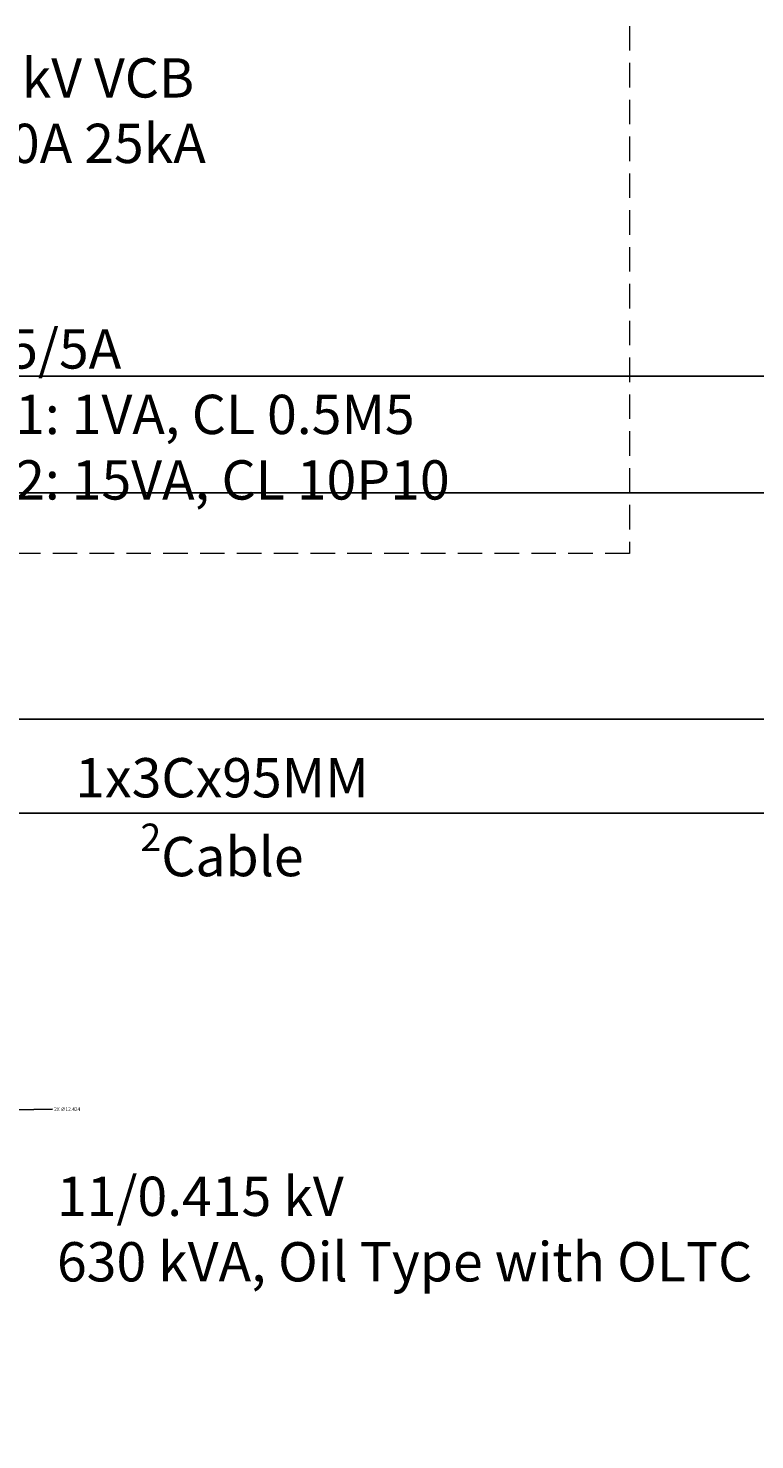
# Model space of a CAD drawing. Units: inches. Extents: x 412 to 584, y 208 to 437.
# Tile 21 of 28: x 508 to 545, y 315 to 387. Entities that reach past the tile are written whole.
import ezdxf

# ---------------------------------------------------------------- set-up
doc = ezdxf.new("R2010")
doc.units = ezdxf.units.IN
doc.header["$MEASUREMENT"] = 0
doc.linetypes.add('HIDDEN', pattern=[0.375, 0.25, -0.125])
for name, color, linetype, lineweight in [('A-ANNO-DIMS', 2, 'Continuous', 18), ('E-ANNO-TEXT', 7, 'Continuous', 18), ('E-ENCL-HIDN', 3, 'HIDDEN', 18)]:
    doc.layers.add(name, color=color, linetype=linetype, lineweight=lineweight)
doc.styles.get("Standard").update_dxf_attribs({"font": 'arial.ttf'})
doc.dimstyles.get("Standard").update_dxf_attribs({"dimtxt": 0.18, "dimasz": 0.18, "dimexe": 0.18, "dimexo": 0.0625, "dimgap": 0.09, "dimtad": 0, "dimtih": 1, "dimtoh": 1, "dimdec": 4, "dimzin": 0, "dimdsep": 46, "dimtxsty": 'Standard', "dimcen": 0.09, "dimadec": 0, "dimazin": 0, "dimtfac": 1, "dimtdec": 4, "dimtofl": 0, "dimtmove": 0, "dimatfit": 3, "dimfxl": 1, "dimtolj": 1, "dimtzin": 0, "dimarcsym": 0})

# ---------------------------------------------------------------- blocks, each defined once
blk = doc.blocks.new('*D17')
at = {"layer": 'A-ANNO-DIMS', "color": 0, "lineweight": -2, "transparency": 16777216}
for p, q in [((497.715, 426.185), (583.674, 426.185)), ((583.494, 426.005), (583.494, 323.031)), ((583.494, 219.693), (583.494, 322.667)), ((550.198, 219.513), (583.674, 219.513))]:
    blk.add_line(p, q, dxfattribs=at)
at = {"layer": 'A-ANNO-DIMS', "color": 0, "transparency": 16777216}
for points in [[(583.464, 426.005), (583.524, 426.005), (583.494, 426.185)], [(583.464, 219.693), (583.524, 219.693), (583.494, 219.513)]]:
    blk.add_solid(points, dxfattribs=at)
at = {"layer": 'Defpoints', "color": 0, "transparency": 16777216}
for p in [(497.652, 426.185), (550.135, 219.513), (583.494, 219.513)]:
    blk.add_point(p, dxfattribs=at)
at = {"layer": 'A-ANNO-DIMS', "color": 0, "transparency": 16777216, "insert": (583.494, 322.849), "char_height": 0.18, "attachment_point": 5}
blk.add_mtext('\\A1;206.67', dxfattribs=at)
blk = doc.blocks.new('*D28')
at = {"layer": 'A-ANNO-DIMS', "color": 0, "lineweight": -2, "transparency": 16777216}
for p, q in [((450.562, 256.635), (450.562, 437.465)), ((450.742, 437.285), (502.724, 437.285)), ((555.616, 437.285), (503.634, 437.285)), ((555.796, 256.635), (555.796, 437.465))]:
    blk.add_line(p, q, dxfattribs=at)
at = {"layer": 'A-ANNO-DIMS', "color": 0, "transparency": 16777216}
for points in [[(450.742, 437.315), (450.742, 437.255), (450.562, 437.285)], [(555.616, 437.315), (555.616, 437.255), (555.796, 437.285)]]:
    blk.add_solid(points, dxfattribs=at)
at = {"layer": 'Defpoints', "color": 0, "transparency": 16777216}
for p in [(555.796, 437.285), (450.562, 256.573), (555.796, 256.573)]:
    blk.add_point(p, dxfattribs=at)
at = {"layer": 'A-ANNO-DIMS', "color": 0, "transparency": 16777216, "insert": (503.179, 437.285), "char_height": 0.18, "attachment_point": 5}
blk.add_mtext('\\A1;105.23', dxfattribs=at)
blk = doc.blocks.new('*D35')
at = {"layer": 'A-ANNO-DIMS', "color": 0, "lineweight": -2, "transparency": 16777216}
for p, q in [((485.523, 369.221), (583.674, 369.221)), ((583.494, 369.041), (583.494, 366.437)), ((583.494, 363.469), (583.494, 366.073)), ((485.523, 363.289), (583.674, 363.289))]:
    blk.add_line(p, q, dxfattribs=at)
at = {"layer": 'A-ANNO-DIMS', "color": 0, "transparency": 16777216}
for points in [[(583.464, 369.041), (583.524, 369.041), (583.494, 369.221)], [(583.464, 363.469), (583.524, 363.469), (583.494, 363.289)]]:
    blk.add_solid(points, dxfattribs=at)
at = {"layer": 'Defpoints', "color": 0, "transparency": 16777216}
for p in [(485.46, 369.221), (485.46, 363.289), (583.494, 363.289)]:
    blk.add_point(p, dxfattribs=at)
at = {"layer": 'A-ANNO-DIMS', "color": 0, "transparency": 16777216, "insert": (583.494, 366.255), "char_height": 0.18, "attachment_point": 5}
blk.add_mtext('\\A1;5.932', dxfattribs=at)
blk = doc.blocks.new('*D40')
at = {"layer": 'A-ANNO-DIMS', "color": 0, "lineweight": -2, "transparency": 16777216}
for p, q in [((501.747, 351.77), (583.674, 351.77)), ((583.494, 351.59), (583.494, 349.555)), ((583.494, 347.157), (583.494, 349.191)), ((501.747, 346.977), (583.674, 346.977))]:
    blk.add_line(p, q, dxfattribs=at)
at = {"layer": 'A-ANNO-DIMS', "color": 0, "transparency": 16777216}
for points in [[(583.464, 351.59), (583.524, 351.59), (583.494, 351.77)], [(583.464, 347.157), (583.524, 347.157), (583.494, 346.977)]]:
    blk.add_solid(points, dxfattribs=at)
at = {"layer": 'Defpoints', "color": 0, "transparency": 16777216}
for p in [(501.685, 351.77), (501.685, 346.977), (583.494, 346.977)]:
    blk.add_point(p, dxfattribs=at)
at = {"layer": 'A-ANNO-DIMS', "color": 0, "transparency": 16777216, "insert": (583.494, 349.373), "char_height": 0.18, "attachment_point": 5}
blk.add_mtext('\\A1;4.794', dxfattribs=at)
blk = doc.blocks.new('*D42')
at = {"layer": 'A-ANNO-DIMS', "color": 0, "lineweight": -2, "transparency": 16777216}
for p, q in [((499.198, 331.75), (499.378, 331.75)), ((499.288, 331.66), (499.288, 331.84)), ((509.226, 331.91), (505.679, 331.853))]:
    blk.add_line(p, q, dxfattribs=at)
at = {"layer": 'A-ANNO-DIMS', "color": 0, "transparency": 16777216}
blk.add_solid([(505.679, 331.883), (505.68, 331.823), (505.499, 331.85)], dxfattribs=at)
at = {"layer": 'Defpoints', "color": 0, "transparency": 16777216}
for p in [(493.077, 331.649), (505.499, 331.85)]:
    blk.add_point(p, dxfattribs=at)
at = {"layer": 'A-ANNO-DIMS', "color": 0, "transparency": 16777216, "insert": (509.977, 331.91), "char_height": 0.18, "attachment_point": 5}
blk.add_mtext('\\A1;2X ∅12.424', dxfattribs=at)

msp = doc.modelspace()

# ---------------------------------------------------------------- linework, layer by layer
at = {"layer": 'E-ENCL-HIDN', "ltscale": 5}
msp.add_lwpolyline([(466.1037, 400.175), (538.6186, 400.175), (538.6186, 360.1961), (466.1037, 360.1961)], close=True, dxfattribs=at)

# ---------------------------------------------------------------- texts
at = {"layer": 'E-ANNO-TEXT', "char_height": 2, "attachment_point": 1}
for s, width, heights, insert in [('\\pxqc;11kV VCB\\P230A 25kA', 15.674937, [6.8044], (502.7, 385.4105)), ('\\pxql;CT\\P150/5/5A\\PCore1: 1VA, CL 0.5M5\\PCore2: 15VA, CL 10P10', 41.457397, [15.3449], (501.3634, 374.947)), ('\\A1;\\pxqc;1x3Cx95MM{\\H0.7x;\\S2^ ;}Cable', 13.633448, [2.9648], (511.0448, 349.7839)), ('\\pxql;11/0.415 kV\\P630 kVA, Oil Type with OLTC', 37.930034, [8.6192], (509.4585, 328.4764))]:
    msp.add_mtext_dynamic_manual_height_columns(s, width=width, gutter_width=1, heights=heights, dxfattribs=dict(at, insert=insert))

# ---------------------------------------------------------------- dimensions: what is measured, and where the dimension line sits
at = {"layer": 'A-ANNO-DIMS'}
dim = msp.add_linear_dim(base=(555.7959, 437.2847), p1=(450.562, 256.5729), p2=(555.7959, 256.5729), dimstyle='Standard', override={"dimdec": 2, "dimlfac": 1, "dimrnd": 0, "dimzin": 0, "dimdsep": 46, "dimlunit": 2}, dxfattribs=at)
dim.commit()
dim.dimension.update_dxf_attribs({"geometry": '*D28', "text_midpoint": (503.1789, 437.2847)})
for base, p1, p2, override, picture, middle in [((583.4937, 219.5133), (497.6523, 426.1847), (550.1351, 219.5133), {"dimdec": 2, "dimlfac": 1, "dimrnd": 0, "dimzin": 0, "dimdsep": 46, "dimlunit": 2}, '*D17', (583.4937, 322.849)), ((583.4937, 363.2888), (485.4605, 369.221), (485.4605, 363.2888), {"dimdec": 3, "dimlfac": 1, "dimrnd": 0, "dimzin": 0, "dimdsep": 46, "dimlunit": 2}, '*D35', (583.4937, 366.2549)), ((583.4937, 346.9765), (501.6846, 351.7702), (501.6846, 346.9765), {"dimdec": 3, "dimlfac": 1, "dimrnd": 0, "dimzin": 0, "dimdsep": 46, "dimlunit": 2}, '*D40', (583.4937, 349.3734))]:
    dim = msp.add_linear_dim(base=base, p1=p1, p2=p2, angle=90, dimstyle='Standard', override=override, dxfattribs=at)
    dim.commit()
    dim.dimension.update_dxf_attribs({"geometry": picture, "text_midpoint": middle})
dim = msp.add_diameter_dim_2p(p1=(493.0765, 331.6491), p2=(505.4991, 331.8501), text='2X <>', dimstyle='Standard', override={"dimdec": 3, "dimlfac": 1, "dimrnd": 0, "dimzin": 0, "dimdsep": 46, "dimlunit": 2}, dxfattribs=at)
dim.commit()
dim.dimension.update_dxf_attribs({"geometry": '*D42', "text_midpoint": (509.2259, 331.9105), "dimtype": 163})

doc.saveas('drawing.dxf')
